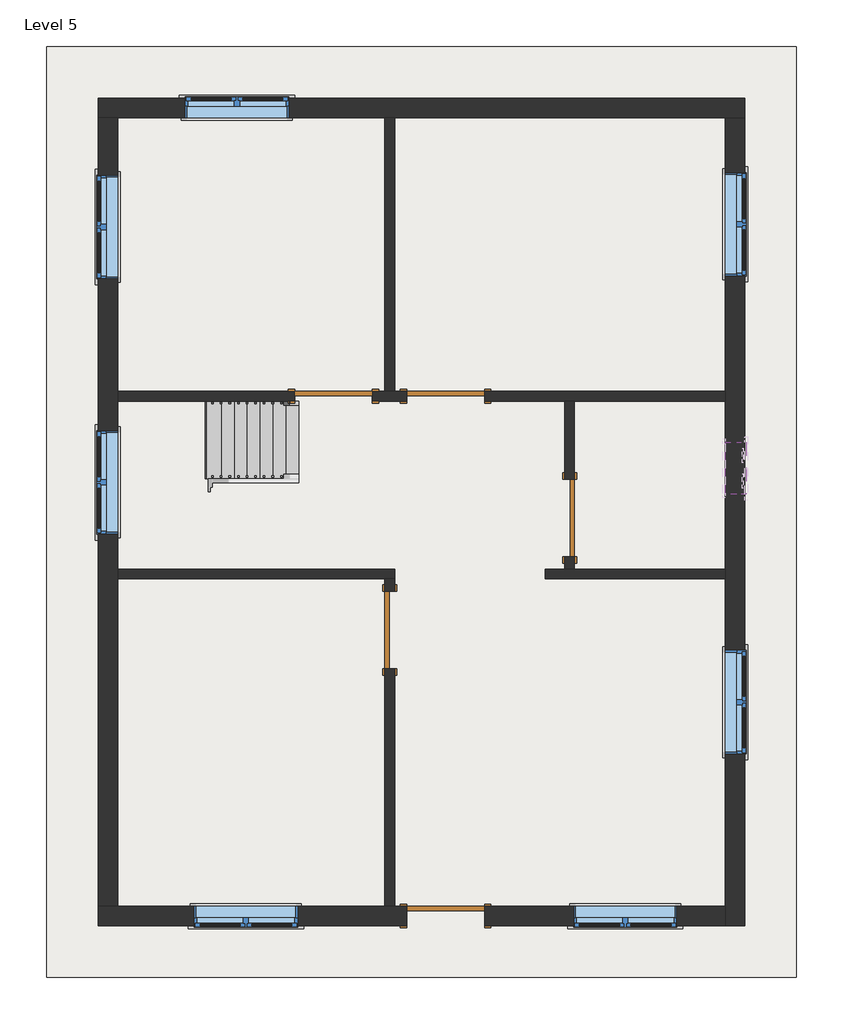
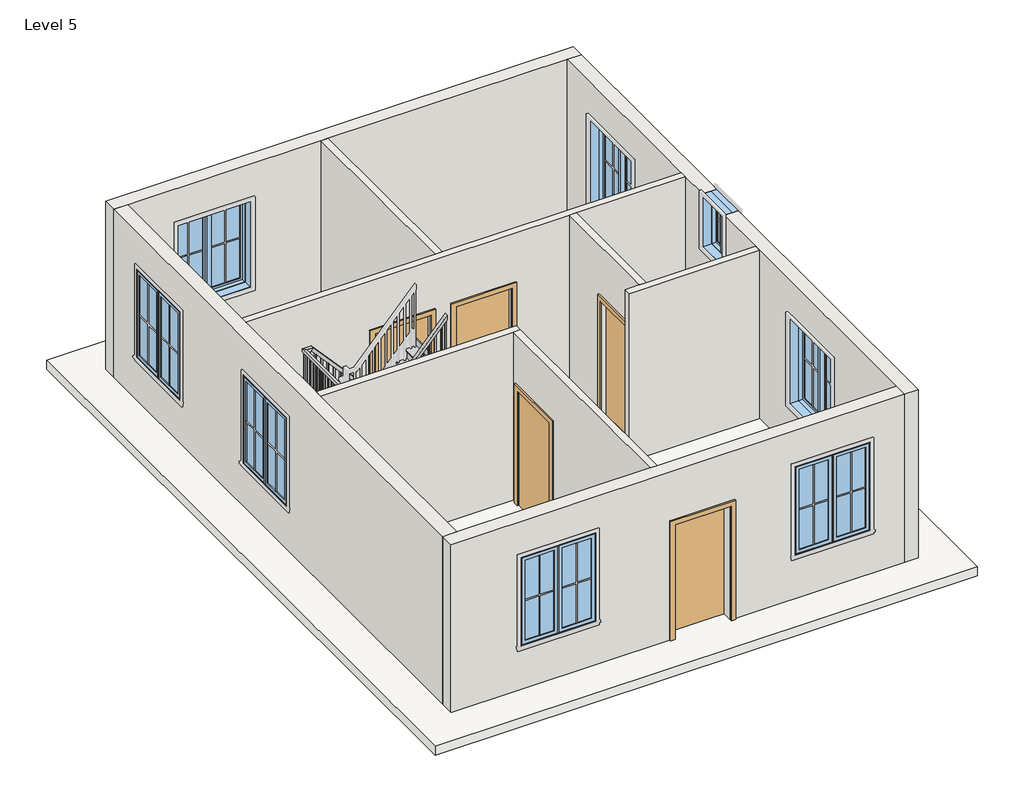
# One storey, part 1 of 2: 10 walls, 8 windows, 5 doors, 1 railing, 1 roof, 1 stair flight.
"""IFC4 building model written with IfcOpenShell, lengths in millimetres."""

from ifc_helpers import new_model, si_unit, frame, origin, place, context, project, spatial, polyline, outline, extrude, faceted_brep, transform, mapped, element, save
from components import door_e5f9f3c4, door_305aa2a5, door_a90ba1ad, stair_flight_93877f9a, window_c417fced, window_8377141f

model = new_model("IFC4")

# Units and contexts
model_context = context("Model", 3, world=origin())
ifc_project = project(units=[si_unit("LENGTHUNIT", "METRE", prefix="MILLI")], contexts=[model_context])

# Site, building, storey
site = spatial("IfcSite", under=ifc_project)
building = spatial("IfcBuilding", under=site)
storey = spatial("IfcBuildingStorey", under=building, Name="Level 5", Elevation=12192.0)

# Doors
placement = place(None, origin())
door_shape = door_e5f9f3c4(model_context)
element("IfcDoor", 1, ObjectType="Single-Flush : 36\" x 84\"", at=placement, inside=storey, context=model_context, shape_type="MappedRepresentation", body=[
    mapped(door_shape, transform((4044.95, 10966.45, 12192.0), x_axis=(1.0, 0.0, 0.0), y_axis=(0.0, 1.0, 0.0), z_axis=(0.0, 0.0, 1.0))),
])
element("IfcDoor", 2, ObjectType="Single-Flush : 36\" x 84\"", at=placement, inside=storey, context=model_context, shape_type="MappedRepresentation", body=[
    mapped(door_shape, transform((4705.35, 8210.55, 12192.0), x_axis=(0.0, 1.0, 0.0), y_axis=(-1.0, 0.0, 0.0), z_axis=(0.0, 0.0, 1.0))),
])
element("IfcDoor", 3, ObjectType="Single-Flush : 36\" x 84\"", at=placement, inside=storey, context=model_context, shape_type="MappedRepresentation", body=[
    mapped(door_shape, transform((6826.25, 9531.35, 12192.0), x_axis=(0.0, -1.0, 0.0), y_axis=(1.0, 0.0, 0.0), z_axis=(0.0, 0.0, 1.0))),
])
door_2_shape = door_305aa2a5(model_context)
element("IfcDoor", 4, ObjectType="Single-Flush : 36\" x 84\"", at=placement, inside=storey, context=model_context, shape_type="MappedRepresentation", body=[
    mapped(door_2_shape, transform((5365.75, 10966.45, 12192.0), x_axis=(-1.0, 0.0, 0.0), y_axis=(0.0, -1.0, 0.0), z_axis=(0.0, 0.0, 1.0))),
])
door_3_shape = door_a90ba1ad(model_context)
element("IfcDoor", 5, ObjectType="Single-Flush : 36\" x 84\"", at=placement, inside=storey, context=model_context, shape_type="MappedRepresentation", body=[
    mapped(door_3_shape, transform((5365.75, 4838.7, 12192.0), x_axis=(-1.0, 0.0, 0.0), y_axis=(0.0, -1.0, 0.0), z_axis=(0.0, 0.0, 1.0))),
])

# Railing
element("IfcRailing", 6, ObjectType="Handrail - Rectangular", at=placement, inside=storey, context=model_context, shape_type="SolidModel", body=[
    faceted_brep([(3632.2, 10858.5, 13275.7333333), (3632.2, 10858.5, 13199.7950998), (3632.2, 10909.3, 13199.7950998), (3632.2, 10909.3, 13275.7333333), (2565.4, 10858.5, 14461.0666667), (2542.7755898, 10858.5, 14410.2666667), (2542.7755898, 10909.3, 14410.2666667), (2565.4, 10909.3, 14461.0666667), (2463.8, 10858.5, 14461.0666667), (2463.8, 10858.5, 14410.2666667), (2413.0, 10909.3, 14410.2666667), (2413.0, 10909.3, 14461.0666667), (2463.8, 9055.1, 14461.0666667), (2463.8, 9004.3, 14410.2666667), (2413.0, 9004.3, 14410.2666667), (2413.0, 9055.1, 14461.0666667), (2463.8, 9055.1, 14602.1777778), (2463.8, 9004.3, 14551.3777778), (2413.0, 9004.3, 14551.3777778), (2413.0, 9055.1, 14602.1777778), (2463.8, 8978.9, 14602.1777778), (2463.8, 8978.9, 14551.3777778), (2413.0, 8928.1, 14551.3777778), (2413.0, 8928.1, 14602.1777778), (2540.0, 8978.9, 14602.1777778), (2562.6244102, 8978.9, 14551.3777778), (2562.6244102, 8928.1, 14551.3777778), (2540.0, 8928.1, 14602.1777778), (3632.2, 8978.9, 15815.7333333), (3632.2, 8928.1, 15815.7333333), (3632.2, 8928.1, 15739.7950998), (3632.2, 8978.9, 15739.7950998)], [[[0, 1, 2, 3]], [[1, 0, 4, 5]], [[2, 1, 5, 6]], [[3, 2, 6, 7]], [[0, 3, 7, 4]], [[5, 4, 8, 9]], [[6, 5, 9, 10]], [[7, 6, 10, 11]], [[4, 7, 11, 8]], [[9, 8, 12, 13]], [[10, 9, 13, 14]], [[11, 10, 14, 15]], [[8, 11, 15, 12]], [[13, 12, 16, 17]], [[14, 13, 17, 18]], [[15, 14, 18, 19]], [[12, 15, 19, 16]], [[17, 16, 20, 21]], [[18, 17, 21, 22]], [[19, 18, 22, 23]], [[16, 19, 23, 20]], [[21, 20, 24, 25]], [[22, 21, 25, 26]], [[23, 22, 26, 27]], [[20, 23, 27, 24]], [[28, 29, 30, 31]], [[25, 24, 28, 31]], [[26, 25, 31, 30]], [[27, 26, 30, 29]], [[24, 27, 29, 28]]]),
    extrude(outline(polyline([(15665.7117665, 3565.525), (15644.5450998, 3546.475), (14732.0, 3546.475), (14732.0, 3565.525), (15665.7117665, 3565.525)])), frame((0.0, 8943.975, 0.0), z_axis=(0.0, 1.0, 0.0), x_axis=(0.0, 0.0, 1.0)), (0.0, 0.0, 1.0), 19.05),
    extrude(outline(polyline([(15552.8228776, 3463.925), (15531.6562109, 3444.875), (14562.6666667, 3444.875), (14562.6666667, 3463.925), (15552.8228776, 3463.925)])), frame((0.0, 8943.975, 0.0), z_axis=(0.0, 1.0, 0.0), x_axis=(0.0, 0.0, 1.0)), (0.0, 0.0, 1.0), 19.05),
    extrude(outline(polyline([(15439.9339887, 3362.325), (15418.767322, 3343.275), (14562.6666667, 3343.275), (14562.6666667, 3362.325), (15439.9339887, 3362.325)])), frame((0.0, 8943.975, 0.0), z_axis=(0.0, 1.0, 0.0), x_axis=(0.0, 0.0, 1.0)), (0.0, 0.0, 1.0), 19.05),
    extrude(outline(polyline([(15327.0450998, 3260.725), (15305.8784332, 3241.675), (14393.3333333, 3241.675), (14393.3333333, 3260.725), (15327.0450998, 3260.725)])), frame((0.0, 8943.975, 0.0), z_axis=(0.0, 1.0, 0.0), x_axis=(0.0, 0.0, 1.0)), (0.0, 0.0, 1.0), 19.05),
    extrude(outline(polyline([(15214.1562109, 3159.125), (15192.9895443, 3140.075), (14224.0, 3140.075), (14224.0, 3159.125), (15214.1562109, 3159.125)])), frame((0.0, 8943.975, 0.0), z_axis=(0.0, 1.0, 0.0), x_axis=(0.0, 0.0, 1.0)), (0.0, 0.0, 1.0), 19.05),
    extrude(outline(polyline([(15101.267322, 3057.525), (15080.1006554, 3038.475), (14224.0, 3038.475), (14224.0, 3057.525), (15101.267322, 3057.525)])), frame((0.0, 8943.975, 0.0), z_axis=(0.0, 1.0, 0.0), x_axis=(0.0, 0.0, 1.0)), (0.0, 0.0, 1.0), 19.05),
    extrude(outline(polyline([(14988.3784332, 2955.925), (14967.2117665, 2936.875), (14054.6666667, 2936.875), (14054.6666667, 2955.925), (14988.3784332, 2955.925)])), frame((0.0, 8943.975, 0.0), z_axis=(0.0, 1.0, 0.0), x_axis=(0.0, 0.0, 1.0)), (0.0, 0.0, 1.0), 19.05),
    extrude(outline(polyline([(14875.4895443, 2854.325), (14854.3228776, 2835.275), (13885.3333333, 2835.275), (13885.3333333, 2854.325), (14875.4895443, 2854.325)])), frame((0.0, 8943.975, 0.0), z_axis=(0.0, 1.0, 0.0), x_axis=(0.0, 0.0, 1.0)), (0.0, 0.0, 1.0), 19.05),
    extrude(outline(polyline([(14762.6006554, 2752.725), (14741.4339887, 2733.675), (13885.3333333, 2733.675), (13885.3333333, 2752.725), (14762.6006554, 2752.725)])), frame((0.0, 8943.975, 0.0), z_axis=(0.0, 1.0, 0.0), x_axis=(0.0, 0.0, 1.0)), (0.0, 0.0, 1.0), 19.05),
    extrude(outline(polyline([(14649.7117665, 2651.125), (14628.5450998, 2632.075), (13716.0, 2632.075), (13716.0, 2651.125), (14649.7117665, 2651.125)])), frame((0.0, 8943.975, 0.0), z_axis=(0.0, 1.0, 0.0), x_axis=(0.0, 0.0, 1.0)), (0.0, 0.0, 1.0), 19.05),
    extrude(outline(polyline([(14536.8228776, 2549.525), (14515.6562109, 2530.475), (13546.6666667, 2530.475), (13546.6666667, 2549.525), (14536.8228776, 2549.525)])), frame((0.0, 8943.975, 0.0), z_axis=(0.0, 1.0, 0.0), x_axis=(0.0, 0.0, 1.0)), (0.0, 0.0, 1.0), 19.05),
    extrude(outline(polyline([(2428.875, 9064.625), (2447.925, 9064.625), (2447.925, 9045.575), (2428.875, 9045.575), (2428.875, 9064.625)])), frame((0.0, 0.0, 13546.6666667), z_axis=(0.0, 0.0, 1.0), x_axis=(1.0, 0.0, 0.0)), (0.0, 0.0, 1.0), 863.6),
    extrude(outline(polyline([(2428.875, 9166.225), (2447.925, 9166.225), (2447.925, 9147.175), (2428.875, 9147.175), (2428.875, 9166.225)])), frame((0.0, 0.0, 13546.6666667), z_axis=(0.0, 0.0, 1.0), x_axis=(1.0, 0.0, 0.0)), (0.0, 0.0, 1.0), 863.6),
    extrude(outline(polyline([(2428.875, 9267.825), (2447.925, 9267.825), (2447.925, 9248.775), (2428.875, 9248.775), (2428.875, 9267.825)])), frame((0.0, 0.0, 13546.6666667), z_axis=(0.0, 0.0, 1.0), x_axis=(1.0, 0.0, 0.0)), (0.0, 0.0, 1.0), 863.6),
    extrude(outline(polyline([(2428.875, 9369.425), (2447.925, 9369.425), (2447.925, 9350.375), (2428.875, 9350.375), (2428.875, 9369.425)])), frame((0.0, 0.0, 13546.6666667), z_axis=(0.0, 0.0, 1.0), x_axis=(1.0, 0.0, 0.0)), (0.0, 0.0, 1.0), 863.6),
    extrude(outline(polyline([(2428.875, 9471.025), (2447.925, 9471.025), (2447.925, 9451.975), (2428.875, 9451.975), (2428.875, 9471.025)])), frame((0.0, 0.0, 13546.6666667), z_axis=(0.0, 0.0, 1.0), x_axis=(1.0, 0.0, 0.0)), (0.0, 0.0, 1.0), 863.6),
    extrude(outline(polyline([(2428.875, 9572.625), (2447.925, 9572.625), (2447.925, 9553.575), (2428.875, 9553.575), (2428.875, 9572.625)])), frame((0.0, 0.0, 13546.6666667), z_axis=(0.0, 0.0, 1.0), x_axis=(1.0, 0.0, 0.0)), (0.0, 0.0, 1.0), 863.6),
    extrude(outline(polyline([(2428.875, 9674.225), (2447.925, 9674.225), (2447.925, 9655.175), (2428.875, 9655.175), (2428.875, 9674.225)])), frame((0.0, 0.0, 13546.6666667), z_axis=(0.0, 0.0, 1.0), x_axis=(1.0, 0.0, 0.0)), (0.0, 0.0, 1.0), 863.6),
    extrude(outline(polyline([(2428.875, 9775.825), (2447.925, 9775.825), (2447.925, 9756.775), (2428.875, 9756.775), (2428.875, 9775.825)])), frame((0.0, 0.0, 13546.6666667), z_axis=(0.0, 0.0, 1.0), x_axis=(1.0, 0.0, 0.0)), (0.0, 0.0, 1.0), 863.6),
    extrude(outline(polyline([(2428.875, 9877.425), (2447.925, 9877.425), (2447.925, 9858.375), (2428.875, 9858.375), (2428.875, 9877.425)])), frame((0.0, 0.0, 13546.6666667), z_axis=(0.0, 0.0, 1.0), x_axis=(1.0, 0.0, 0.0)), (0.0, 0.0, 1.0), 863.6),
    extrude(outline(polyline([(2428.875, 9979.025), (2447.925, 9979.025), (2447.925, 9959.975), (2428.875, 9959.975), (2428.875, 9979.025)])), frame((0.0, 0.0, 13546.6666667), z_axis=(0.0, 0.0, 1.0), x_axis=(1.0, 0.0, 0.0)), (0.0, 0.0, 1.0), 863.6),
    extrude(outline(polyline([(2428.875, 10080.625), (2447.925, 10080.625), (2447.925, 10061.575), (2428.875, 10061.575), (2428.875, 10080.625)])), frame((0.0, 0.0, 13546.6666667), z_axis=(0.0, 0.0, 1.0), x_axis=(1.0, 0.0, 0.0)), (0.0, 0.0, 1.0), 863.6),
    extrude(outline(polyline([(2428.875, 10182.225), (2447.925, 10182.225), (2447.925, 10163.175), (2428.875, 10163.175), (2428.875, 10182.225)])), frame((0.0, 0.0, 13546.6666667), z_axis=(0.0, 0.0, 1.0), x_axis=(1.0, 0.0, 0.0)), (0.0, 0.0, 1.0), 863.6),
    extrude(outline(polyline([(2428.875, 10283.825), (2447.925, 10283.825), (2447.925, 10264.775), (2428.875, 10264.775), (2428.875, 10283.825)])), frame((0.0, 0.0, 13546.6666667), z_axis=(0.0, 0.0, 1.0), x_axis=(1.0, 0.0, 0.0)), (0.0, 0.0, 1.0), 863.6),
    extrude(outline(polyline([(2428.875, 10385.425), (2447.925, 10385.425), (2447.925, 10366.375), (2428.875, 10366.375), (2428.875, 10385.425)])), frame((0.0, 0.0, 13546.6666667), z_axis=(0.0, 0.0, 1.0), x_axis=(1.0, 0.0, 0.0)), (0.0, 0.0, 1.0), 863.6),
    extrude(outline(polyline([(2428.875, 10487.025), (2447.925, 10487.025), (2447.925, 10467.975), (2428.875, 10467.975), (2428.875, 10487.025)])), frame((0.0, 0.0, 13546.6666667), z_axis=(0.0, 0.0, 1.0), x_axis=(1.0, 0.0, 0.0)), (0.0, 0.0, 1.0), 863.6),
    extrude(outline(polyline([(2428.875, 10588.625), (2447.925, 10588.625), (2447.925, 10569.575), (2428.875, 10569.575), (2428.875, 10588.625)])), frame((0.0, 0.0, 13546.6666667), z_axis=(0.0, 0.0, 1.0), x_axis=(1.0, 0.0, 0.0)), (0.0, 0.0, 1.0), 863.6),
    extrude(outline(polyline([(2428.875, 10690.225), (2447.925, 10690.225), (2447.925, 10671.175), (2428.875, 10671.175), (2428.875, 10690.225)])), frame((0.0, 0.0, 13546.6666667), z_axis=(0.0, 0.0, 1.0), x_axis=(1.0, 0.0, 0.0)), (0.0, 0.0, 1.0), 863.6),
    extrude(outline(polyline([(2428.875, 10791.825), (2447.925, 10791.825), (2447.925, 10772.775), (2428.875, 10772.775), (2428.875, 10791.825)])), frame((0.0, 0.0, 13546.6666667), z_axis=(0.0, 0.0, 1.0), x_axis=(1.0, 0.0, 0.0)), (0.0, 0.0, 1.0), 863.6),
    extrude(outline(polyline([(2524.125, 10893.425), (2524.125, 10874.375), (2505.075, 10874.375), (2505.075, 10893.425), (2524.125, 10893.425)])), frame((0.0, 0.0, 13546.6666667), z_axis=(0.0, 0.0, 1.0), x_axis=(1.0, 0.0, 0.0)), (0.0, 0.0, 1.0), 863.6),
    extrude(outline(polyline([(14318.1006554, 2625.725), (14339.267322, 2606.675), (13377.3333333, 2606.675), (13377.3333333, 2625.725), (14318.1006554, 2625.725)])), frame((0.0, 10874.375, 0.0), z_axis=(0.0, 1.0, 0.0), x_axis=(0.0, 0.0, 1.0)), (0.0, 0.0, 1.0), 19.05),
    extrude(outline(polyline([(14205.2117665, 2727.325), (14226.3784332, 2708.275), (13377.3333333, 2708.275), (13377.3333333, 2727.325), (14205.2117665, 2727.325)])), frame((0.0, 10874.375, 0.0), z_axis=(0.0, 1.0, 0.0), x_axis=(0.0, 0.0, 1.0)), (0.0, 0.0, 1.0), 19.05),
    extrude(outline(polyline([(14092.3228776, 2828.925), (14113.4895443, 2809.875), (13208.0, 2809.875), (13208.0, 2828.925), (14092.3228776, 2828.925)])), frame((0.0, 10874.375, 0.0), z_axis=(0.0, 1.0, 0.0), x_axis=(0.0, 0.0, 1.0)), (0.0, 0.0, 1.0), 19.05),
    extrude(outline(polyline([(13979.4339887, 2930.525), (14000.6006554, 2911.475), (13038.6666667, 2911.475), (13038.6666667, 2930.525), (13979.4339887, 2930.525)])), frame((0.0, 10874.375, 0.0), z_axis=(0.0, 1.0, 0.0), x_axis=(0.0, 0.0, 1.0)), (0.0, 0.0, 1.0), 19.05),
    extrude(outline(polyline([(13866.5450998, 3032.125), (13887.7117665, 3013.075), (13038.6666667, 3013.075), (13038.6666667, 3032.125), (13866.5450998, 3032.125)])), frame((0.0, 10874.375, 0.0), z_axis=(0.0, 1.0, 0.0), x_axis=(0.0, 0.0, 1.0)), (0.0, 0.0, 1.0), 19.05),
    extrude(outline(polyline([(13753.6562109, 3133.725), (13774.8228776, 3114.675), (12869.3333333, 3114.675), (12869.3333333, 3133.725), (13753.6562109, 3133.725)])), frame((0.0, 10874.375, 0.0), z_axis=(0.0, 1.0, 0.0), x_axis=(0.0, 0.0, 1.0)), (0.0, 0.0, 1.0), 19.05),
    extrude(outline(polyline([(13640.767322, 3235.325), (13661.9339887, 3216.275), (12700.0, 3216.275), (12700.0, 3235.325), (13640.767322, 3235.325)])), frame((0.0, 10874.375, 0.0), z_axis=(0.0, 1.0, 0.0), x_axis=(0.0, 0.0, 1.0)), (0.0, 0.0, 1.0), 19.05),
    extrude(outline(polyline([(13527.8784332, 3336.925), (13549.0450998, 3317.875), (12700.0, 3317.875), (12700.0, 3336.925), (13527.8784332, 3336.925)])), frame((0.0, 10874.375, 0.0), z_axis=(0.0, 1.0, 0.0), x_axis=(0.0, 0.0, 1.0)), (0.0, 0.0, 1.0), 19.05),
    extrude(outline(polyline([(13414.9895443, 3438.525), (13436.1562109, 3419.475), (12530.6666667, 3419.475), (12530.6666667, 3438.525), (13414.9895443, 3438.525)])), frame((0.0, 10874.375, 0.0), z_axis=(0.0, 1.0, 0.0), x_axis=(0.0, 0.0, 1.0)), (0.0, 0.0, 1.0), 19.05),
    extrude(outline(polyline([(13302.1006554, 3540.125), (13323.267322, 3521.075), (12361.3333333, 3521.075), (12361.3333333, 3540.125), (13302.1006554, 3540.125)])), frame((0.0, 10874.375, 0.0), z_axis=(0.0, 1.0, 0.0), x_axis=(0.0, 0.0, 1.0)), (0.0, 0.0, 1.0), 19.05),
    extrude(outline(polyline([(2428.875, 8963.025), (2447.925, 8963.025), (2447.925, 8943.975), (2428.875, 8943.975), (2428.875, 8963.025)])), frame((0.0, 0.0, 13546.6666667), z_axis=(0.0, 0.0, 1.0), x_axis=(1.0, 0.0, 0.0)), (0.0, 0.0, 1.0), 1004.7111111),
    extrude(outline(polyline([(2447.925, 10893.425), (2447.925, 10874.375), (2428.875, 10874.375), (2428.875, 10893.425), (2447.925, 10893.425)])), frame((0.0, 0.0, 13546.6666667), z_axis=(0.0, 0.0, 1.0), x_axis=(1.0, 0.0, 0.0)), (0.0, 0.0, 1.0), 863.6),
    extrude(outline(polyline([(15739.7950998, 3632.2), (15718.6284332, 3613.15), (14732.0, 3613.15), (14732.0, 3632.2), (15739.7950998, 3632.2)])), frame((0.0, 8943.975, 0.0), z_axis=(0.0, 1.0, 0.0), x_axis=(0.0, 0.0, 1.0)), (0.0, 0.0, 1.0), 19.05),
    extrude(outline(polyline([(13199.7950998, 3632.2), (13220.9617665, 3613.15), (12361.3333333, 3613.15), (12361.3333333, 3632.2), (13199.7950998, 3632.2)])), frame((0.0, 10874.375, 0.0), z_axis=(0.0, 1.0, 0.0), x_axis=(0.0, 0.0, 1.0)), (0.0, 0.0, 1.0), 19.05),
])

# Roof
element("IfcRoof", 7, ObjectType="Generic - 12\"", at=placement, inside=storey, context=model_context, shape_type="SweptSolid", body=[
    extrude(outline(polyline([(660.4, 15087.6), (9499.6, 15087.6), (9499.6, 4114.8), (660.4, 4114.8), (660.4, 15087.6)])), frame((0.0, 0.0, 12192.0), z_axis=(0.0, 0.0, 1.0), x_axis=(1.0, 0.0, 0.0)), (0.0, 0.0, 1.0), 152.4),
])

# Stair flight
stair_flight_shape = stair_flight_93877f9a(model_context)
element("IfcStairFlight", 8, ObjectType="2\" Tread 1\" Nosing 1/4\" Riser", at=placement, inside=storey, context=model_context, shape_type="MappedRepresentation", body=[
    mapped(stair_flight_shape, transform((0.0, 0.0, 0.0), x_axis=(1.0, 0.0, 0.0), y_axis=(0.0, 1.0, 0.0), z_axis=(0.0, 0.0, 1.0))),
])

# Walls
element("IfcWall", 9, ObjectType="Generic - 5\"", at=placement, inside=storey, context=model_context, shape_type="SweptSolid", body=[
    extrude(outline(polyline([(4648.2, 11023.6), (4648.2, 14249.4), (4762.5, 14249.4), (4762.5, 11023.6), (4648.2, 11023.6)])), frame((0.0, 0.0, 12192.0), z_axis=(0.0, 0.0, 1.0), x_axis=(1.0, 0.0, 0.0)), (0.0, 0.0, 1.0), 3048.0),
])
element("IfcWall", 10, ObjectType="Generic - 5\"", at=placement, inside=storey, context=model_context, shape_type="Brep", body=[
    faceted_brep([(4502.15, 10909.3, 12192.0), (4908.55, 10909.3, 12192.0), (4908.55, 10909.3, 14325.6), (5822.95, 10909.3, 14325.6), (5822.95, 10909.3, 12192.0), (6769.1, 10909.3, 12192.0), (6883.4, 10909.3, 12192.0), (8661.4, 10909.3, 12192.0), (8661.4, 10909.3, 15240.0), (6883.4, 10909.3, 15240.0), (6769.1, 10909.3, 15240.0), (1498.6, 10909.3, 15240.0), (1498.6, 10909.3, 12192.0), (3587.75, 10909.3, 12192.0), (3587.75, 10909.3, 14325.6), (4502.15, 10909.3, 14325.6), (4908.55, 11023.6, 14325.6), (4908.55, 11023.6, 12192.0), (4762.5, 11023.6, 12192.0), (4648.2, 11023.6, 12192.0), (4502.15, 11023.6, 12192.0), (4502.15, 11023.6, 14325.6), (3587.75, 11023.6, 14325.6), (3587.75, 11023.6, 12192.0), (1498.6, 11023.6, 12192.0), (1498.6, 11023.6, 15240.0), (4648.2, 11023.6, 15240.0), (4762.5, 11023.6, 15240.0), (8661.4, 11023.6, 15240.0), (8661.4, 11023.6, 12192.0), (5822.95, 11023.6, 12192.0), (5822.95, 11023.6, 14325.6)], [[[0, 1, 2, 3, 4, 5, 6, 7, 8, 9, 10, 11, 12, 13, 14, 15]], [[16, 17, 18, 19, 20, 21, 22, 23, 24, 25, 26, 27, 28, 29, 30, 31]], [[13, 12, 24, 23]], [[30, 29, 7, 6, 5, 4]], [[20, 19, 18, 17, 1, 0]], [[11, 10, 9, 8, 28, 27, 26, 25]], [[8, 7, 29, 28]], [[12, 11, 25, 24]], [[21, 20, 0, 15]], [[22, 21, 15, 14]], [[23, 22, 14, 13]], [[2, 1, 17, 16]], [[3, 2, 16, 31]], [[4, 3, 31, 30]]]),
])
element("IfcWall", 11, ObjectType="Generic - 5\"", at=placement, inside=storey, context=model_context, shape_type="SweptSolid", body=[
    extrude(outline(polyline([(9074.15, 14325.6), (9074.15, 12192.0), (8928.1, 12192.0), (8928.1, 15240.0), (10909.3, 15240.0), (10909.3, 12192.0), (9988.55, 12192.0), (9988.55, 14325.6), (9074.15, 14325.6)])), frame((6769.1, 0.0, 0.0), z_axis=(1.0, 0.0, 0.0), x_axis=(0.0, 1.0, 0.0)), (0.0, 0.0, 1.0), 114.3),
])
element("IfcWall", 12, ObjectType="Generic - 5\"", at=placement, inside=storey, context=model_context, shape_type="Brep", body=[
    faceted_brep([(1498.6, 8813.8, 12192.0), (4648.2, 8813.8, 12192.0), (4762.5, 8813.8, 12192.0), (4762.5, 8813.8, 15240.0), (4648.2, 8813.8, 15240.0), (1498.6, 8813.8, 15240.0), (1498.6, 8928.1, 12192.0), (1498.6, 8928.1, 15240.0), (4762.5, 8928.1, 15240.0), (4762.5, 8928.1, 12192.0)], [[[0, 1, 2, 3, 4, 5]], [[6, 7, 8, 9]], [[2, 1, 0, 6, 9]], [[5, 4, 3, 8, 7]], [[0, 5, 7, 6]], [[3, 2, 9, 8]]]),
])
element("IfcWall", 13, ObjectType="Generic - 5\"", at=placement, inside=storey, context=model_context, shape_type="SweptSolid", body=[
    extrude(outline(polyline([(8813.8, 12192.0), (8667.75, 12192.0), (8667.75, 14325.6), (7753.35, 14325.6), (7753.35, 12192.0), (4953.0, 12192.0), (4953.0, 15240.0), (8813.8, 15240.0), (8813.8, 12192.0)])), frame((4648.2, 0.0, 0.0), z_axis=(1.0, 0.0, 0.0), x_axis=(0.0, 1.0, 0.0)), (0.0, 0.0, 1.0), 114.3),
])
element("IfcWall", 14, ObjectType="Generic - 5\"", at=placement, inside=storey, context=model_context, shape_type="Brep", body=[
    faceted_brep([(6540.5050896, 8813.8, 12192.0), (8661.4, 8813.8, 12192.0), (8661.4, 8813.8, 15240.0), (6540.5050896, 8813.8, 15240.0), (6540.5050896, 8928.1, 12192.0), (6540.5050896, 8928.1, 15240.0), (6769.1, 8928.1, 15240.0), (6883.4, 8928.1, 15240.0), (8661.4, 8928.1, 15240.0), (8661.4, 8928.1, 12192.0), (6883.4, 8928.1, 12192.0), (6769.1, 8928.1, 12192.0)], [[[0, 1, 2, 3]], [[4, 5, 6, 7, 8, 9, 10, 11]], [[1, 0, 4, 11, 10, 9]], [[3, 2, 8, 7, 6, 5]], [[0, 3, 5, 4]], [[2, 1, 9, 8]]]),
])
element("IfcWall", 15, ObjectType="Generic - 8\"", at=placement, inside=storey, context=model_context, shape_type="Brep", body=[
    faceted_brep([(1270.0, 14249.4, 12192.0), (1498.6, 14249.4, 12192.0), (4648.2, 14249.4, 12192.0), (4762.5, 14249.4, 12192.0), (8661.4, 14249.4, 12192.0), (8890.0, 14249.4, 12192.0), (8890.0, 14249.4, 15240.0), (8661.4, 14249.4, 15240.0), (4762.5, 14249.4, 15240.0), (4648.2, 14249.4, 15240.0), (1498.6, 14249.4, 15240.0), (1270.0, 14249.4, 15240.0), (3514.725, 14249.4, 14630.4), (3514.725, 14249.4, 13106.4), (2295.525, 14249.4, 13106.4), (2295.525, 14249.4, 14630.4), (1270.0, 14478.0, 12192.0), (1270.0, 14478.0, 15240.0), (8890.0, 14478.0, 15240.0), (8890.0, 14478.0, 12192.0), (3514.725, 14478.0, 14630.4), (2295.525, 14478.0, 14630.4), (2295.525, 14478.0, 13106.4), (3514.725, 14478.0, 13106.4)], [[[0, 1, 2, 3, 4, 5, 6, 7, 8, 9, 10, 11], [12, 13, 14, 15]], [[16, 17, 18, 19], [20, 21, 22, 23]], [[5, 4, 3, 2, 1, 0, 16, 19]], [[11, 10, 9, 8, 7, 6, 18, 17]], [[6, 5, 19, 18]], [[0, 11, 17, 16]], [[13, 12, 20, 23]], [[14, 13, 23, 22]], [[15, 14, 22, 21]], [[12, 15, 21, 20]]]),
])
element("IfcWall", 16, ObjectType="Generic - 8\"", at=placement, inside=storey, context=model_context, shape_type="Brep", body=[
    faceted_brep([(8661.4, 14249.4, 12192.0), (8661.4, 11023.6, 12192.0), (8661.4, 10909.3, 12192.0), (8661.4, 8928.1, 12192.0), (8661.4, 8813.8, 12192.0), (8661.4, 4953.0, 12192.0), (8661.4, 4724.4, 12192.0), (8661.4, 4724.4, 15240.0), (8661.4, 4953.0, 15240.0), (8661.4, 8813.8, 15240.0), (8661.4, 8928.1, 15240.0), (8661.4, 9810.75, 15240.0), (8661.4, 9810.75, 14325.6), (8661.4, 10420.35, 14325.6), (8661.4, 10420.35, 15240.0), (8661.4, 10909.3, 15240.0), (8661.4, 11023.6, 15240.0), (8661.4, 14249.4, 15240.0), (8661.4, 6750.05, 14630.4), (8661.4, 6750.05, 13106.4), (8661.4, 7969.25, 13106.4), (8661.4, 7969.25, 14630.4), (8661.4, 12382.5, 14630.4), (8661.4, 12382.5, 13106.4), (8661.4, 13601.7, 13106.4), (8661.4, 13601.7, 14630.4), (8890.0, 4724.4, 12192.0), (8890.0, 14249.4, 12192.0), (8890.0, 14249.4, 15240.0), (8890.0, 10420.35, 15240.0), (8890.0, 10420.35, 14325.6), (8890.0, 9810.75, 14325.6), (8890.0, 9810.75, 15240.0), (8890.0, 4724.4, 15240.0), (8890.0, 6750.05, 13106.4), (8890.0, 6750.05, 14630.4), (8890.0, 7969.25, 14630.4), (8890.0, 7969.25, 13106.4), (8890.0, 12382.5, 13106.4), (8890.0, 12382.5, 14630.4), (8890.0, 13601.7, 14630.4), (8890.0, 13601.7, 13106.4)], [[[0, 1, 2, 3, 4, 5, 6, 7, 8, 9, 10, 11, 12, 13, 14, 15, 16, 17], [18, 19, 20, 21], [22, 23, 24, 25]], [[26, 27, 28, 29, 30, 31, 32, 33], [34, 35, 36, 37], [38, 39, 40, 41]], [[6, 5, 4, 3, 2, 1, 0, 27, 26]], [[28, 17, 16, 15, 14, 29]], [[7, 33, 32, 11, 10, 9, 8]], [[0, 17, 28, 27]], [[7, 6, 26, 33]], [[19, 18, 35, 34]], [[20, 19, 34, 37]], [[21, 20, 37, 36]], [[18, 21, 36, 35]], [[23, 22, 39, 38]], [[24, 23, 38, 41]], [[25, 24, 41, 40]], [[22, 25, 40, 39]], [[31, 12, 11, 32]], [[12, 31, 30, 13]], [[13, 30, 29, 14]]]),
])
element("IfcWall", 17, ObjectType="Generic - 8\"", at=placement, inside=storey, context=model_context, shape_type="Brep", body=[
    faceted_brep([(4908.55, 4953.0, 14325.6), (4908.55, 4953.0, 12192.0), (4762.5, 4953.0, 12192.0), (4648.2, 4953.0, 12192.0), (1498.6, 4953.0, 12192.0), (1270.0, 4953.0, 12192.0), (1270.0, 4953.0, 15240.0), (1498.6, 4953.0, 15240.0), (4648.2, 4953.0, 15240.0), (4762.5, 4953.0, 15240.0), (8661.4, 4953.0, 15240.0), (8661.4, 4953.0, 12192.0), (5822.95, 4953.0, 12192.0), (5822.95, 4953.0, 14325.6), (2400.3, 4953.0, 14630.4), (2400.3, 4953.0, 13106.4), (3619.5, 4953.0, 13106.4), (3619.5, 4953.0, 14630.4), (6872.2875, 4953.0, 14630.4), (6872.2875, 4953.0, 13106.4), (8091.4875, 4953.0, 13106.4), (8091.4875, 4953.0, 14630.4), (1270.0, 4724.4, 12192.0), (4908.55, 4724.4, 12192.0), (4908.55, 4724.4, 14325.6), (5822.95, 4724.4, 14325.6), (5822.95, 4724.4, 12192.0), (8661.4, 4724.4, 12192.0), (8661.4, 4724.4, 15240.0), (1270.0, 4724.4, 15240.0), (2400.3, 4724.4, 14630.4), (3619.5, 4724.4, 14630.4), (3619.5, 4724.4, 13106.4), (2400.3, 4724.4, 13106.4), (6872.2875, 4724.4, 14630.4), (8091.4875, 4724.4, 14630.4), (8091.4875, 4724.4, 13106.4), (6872.2875, 4724.4, 13106.4)], [[[0, 1, 2, 3, 4, 5, 6, 7, 8, 9, 10, 11, 12, 13], [14, 15, 16, 17], [18, 19, 20, 21]], [[22, 23, 24, 25, 26, 27, 28, 29], [30, 31, 32, 33], [34, 35, 36, 37]], [[12, 11, 27, 26]], [[5, 4, 3, 2, 1, 23, 22]], [[10, 9, 8, 7, 6, 29, 28]], [[11, 10, 28, 27]], [[6, 5, 22, 29]], [[24, 23, 1, 0]], [[25, 24, 0, 13]], [[26, 25, 13, 12]], [[15, 14, 30, 33]], [[16, 15, 33, 32]], [[17, 16, 32, 31]], [[14, 17, 31, 30]], [[19, 18, 34, 37]], [[20, 19, 37, 36]], [[21, 20, 36, 35]], [[18, 21, 35, 34]]]),
])
element("IfcWall", 18, ObjectType="Generic - 8\"", at=placement, inside=storey, context=model_context, shape_type="Brep", body=[
    faceted_brep([(1498.6, 4953.0, 12192.0), (1498.6, 8813.8, 12192.0), (1498.6, 8928.1, 12192.0), (1498.6, 10909.3, 12192.0), (1498.6, 11023.6, 12192.0), (1498.6, 14249.4, 12192.0), (1498.6, 14249.4, 15240.0), (1498.6, 11023.6, 15240.0), (1498.6, 10909.3, 15240.0), (1498.6, 8928.1, 15240.0), (1498.6, 8813.8, 15240.0), (1498.6, 4953.0, 15240.0), (1498.6, 13569.95, 14630.4), (1498.6, 13569.95, 13106.4), (1498.6, 12350.75, 13106.4), (1498.6, 12350.75, 14630.4), (1498.6, 10560.05, 14630.4), (1498.6, 10560.05, 13106.4), (1498.6, 9340.85, 13106.4), (1498.6, 9340.85, 14630.4), (1270.0, 14249.4, 12192.0), (1270.0, 4953.0, 12192.0), (1270.0, 4953.0, 15240.0), (1270.0, 14249.4, 15240.0), (1270.0, 13569.95, 13106.4), (1270.0, 13569.95, 14630.4), (1270.0, 12350.75, 14630.4), (1270.0, 12350.75, 13106.4), (1270.0, 10560.05, 13106.4), (1270.0, 10560.05, 14630.4), (1270.0, 9340.85, 14630.4), (1270.0, 9340.85, 13106.4)], [[[0, 1, 2, 3, 4, 5, 6, 7, 8, 9, 10, 11], [12, 13, 14, 15], [16, 17, 18, 19]], [[20, 21, 22, 23], [24, 25, 26, 27], [28, 29, 30, 31]], [[5, 4, 3, 2, 1, 0, 21, 20]], [[11, 10, 9, 8, 7, 6, 23, 22]], [[6, 5, 20, 23]], [[0, 11, 22, 21]], [[13, 12, 25, 24]], [[14, 13, 24, 27]], [[15, 14, 27, 26]], [[12, 15, 26, 25]], [[17, 16, 29, 28]], [[18, 17, 28, 31]], [[19, 18, 31, 30]], [[16, 19, 30, 29]]]),
])

# Windows
window_shape = window_c417fced(model_context)
element("IfcWindow", 19, ObjectType="Window-Casement-Double : 24\" x 36\"", at=placement, inside=storey, context=model_context, shape_type="MappedRepresentation", body=[
    mapped(window_shape, transform((8775.7, 10115.55, 13411.2), x_axis=(0.0, -1.0, 0.0), y_axis=(1.0, 0.0, 0.0), z_axis=(0.0, 0.0, 1.0))),
])
window_2_shape = window_8377141f(model_context)
element("IfcWindow", 20, ObjectType="Window-Casement-Double : 48\" x 60\"", at=placement, inside=storey, context=model_context, shape_type="MappedRepresentation", body=[
    mapped(window_2_shape, transform((7481.8875, 4838.7, 12192.0), x_axis=(-1.0, 0.0, 0.0), y_axis=(0.0, -1.0, 0.0), z_axis=(0.0, 0.0, 1.0))),
])
element("IfcWindow", 21, ObjectType="Window-Casement-Double : 48\" x 60\"", at=placement, inside=storey, context=model_context, shape_type="MappedRepresentation", body=[
    mapped(window_2_shape, transform((3009.9, 4838.7, 12192.0), x_axis=(-1.0, 0.0, 0.0), y_axis=(0.0, -1.0, 0.0), z_axis=(0.0, 0.0, 1.0))),
])
element("IfcWindow", 22, ObjectType="Window-Casement-Double : 48\" x 60\"", at=placement, inside=storey, context=model_context, shape_type="MappedRepresentation", body=[
    mapped(window_2_shape, transform((8775.7, 12992.1, 12192.0), x_axis=(0.0, -1.0, 0.0), y_axis=(1.0, 0.0, 0.0), z_axis=(0.0, 0.0, 1.0))),
])
element("IfcWindow", 23, ObjectType="Window-Casement-Double : 48\" x 60\"", at=placement, inside=storey, context=model_context, shape_type="MappedRepresentation", body=[
    mapped(window_2_shape, transform((8775.7, 7359.65, 12192.0), x_axis=(0.0, -1.0, 0.0), y_axis=(1.0, 0.0, 0.0), z_axis=(0.0, 0.0, 1.0))),
])
element("IfcWindow", 24, ObjectType="Window-Casement-Double : 48\" x 60\"", at=placement, inside=storey, context=model_context, shape_type="MappedRepresentation", body=[
    mapped(window_2_shape, transform((1384.3, 12960.35, 12192.0), x_axis=(0.0, 1.0, 0.0), y_axis=(-1.0, 0.0, 0.0), z_axis=(0.0, 0.0, 1.0))),
])
element("IfcWindow", 25, ObjectType="Window-Casement-Double : 48\" x 60\"", at=placement, inside=storey, context=model_context, shape_type="MappedRepresentation", body=[
    mapped(window_2_shape, transform((1384.3, 9950.45, 12192.0), x_axis=(0.0, 1.0, 0.0), y_axis=(-1.0, 0.0, 0.0), z_axis=(0.0, 0.0, 1.0))),
])
element("IfcWindow", 26, ObjectType="Window-Casement-Double : 48\" x 60\"", at=placement, inside=storey, context=model_context, shape_type="MappedRepresentation", body=[
    mapped(window_2_shape, transform((2905.125, 14363.7, 12192.0), x_axis=(1.0, 0.0, 0.0), y_axis=(0.0, 1.0, 0.0), z_axis=(0.0, 0.0, 1.0))),
])

save(model, "model.ifc")

# Revit data of these elements
# Type "Single-Flush : 36\" x 84\""
#   Type Mark = "1"
#   Construction Type Id = "MDOOR"
#   Assembly Code = "C1020"
#   Analytic Construction = "Metal"
#   Thickness = 0' - 2"
#   Heat Transfer Coefficient (U) = 0.651978 BTU/(h·ft²·°F)
#   Height = 7' - 0"
#   Trim Projection Ext = 0' - 1"
#   Trim Projection Int = 0' - 1"
#   Trim Width = 0' - 3"
#   Width = 3' - 0"
#   Define Thermal Properties by = 1
#   Define Thermal Properties by = 1
#   Door Material = Door - Panel
#   Frame Material = Door - Frame
#   Visual Light Transmittance = 0
#   Solar Heat Gain Coefficient = 0
#   Function = (empty or 0)
#   Wall Closure = (empty or 0)
# Type "Handrail - Rectangular"
#   Assembly Code = "C2010400"
#   built-in parameter 1008612 = 0.0416667 (stored number, unit not read)
#   built-in parameter 1008611 = 0.0416667 (stored number, unit not read)
#   built-in parameter 1008609 = 0.333333 (stored number, unit not read)
#   built-in parameter 1008604 = 0.166667 (stored number, unit not read)
#   built-in parameter 1008603 = 0.166667 (stored number, unit not read)
#   Railing Height = 3' - 0"
#   built-in parameter 1008630 = 2
#   built-in parameter 1008610 = 2
#   built-in parameter 1008618 = Baluster - Square : 3/4"
# Type "Generic - 12\""
#   Assembly Code = "B1020"
#   Layers, outside or top first: 0' - 6" no material (function 1)
# Type "Generic - 5\""
#   Assembly Code = "B2010"
#   Layers, outside or top first: 0' - 4 1/2" no material (function 1)
# Type "Generic - 8\""
#   Assembly Code = "B2010"
#   Layers, outside or top first: 0' - 9" "Parking Stripe" (function 1)
# Type "Window-Casement-Double : 24\" x 36\""
#   Type Mark = "14"
#   Fire Rating = "0.5h"
#   Assembly Code = "B2020100"
#   Analytic Construction = "Double glazing - domestic"
#   Frame Extension [instance default] = 0' - 0 1/4"
#   Window Inset [instance default] = 0' - 0"
#   Wall Thickness [instance default] = 0' - 6"
#   Interior Wall Closure [instance default] = 0' - 2 1/4"
#   Half Width = 1' - 0"
#   Visual Light Transmittance = 0.81
#   Thermal Resistance (R) = 1.8146 (h·ft²·°F)/BTU
#   Solar Heat Gain Coefficient = 0.76
#   Rough Width = 2' - 0 1/2"
#   Rough Height = 3' - 0 1/2"
#   Height = 3' - 0"
#   Heat Transfer Coefficient (U) = 0.5511 BTU/(h·ft²·°F)
#   Exterior Wall Closure [instance default] = 0' - 1 1/4"
#   Extension Jamb [instance default] = 0' - 2 1/4"
#   Default Sill Height = 3' - 0"
#   Width = 2' - 0"
#   Define Thermal Properties by = 0
#   Muntin Visibility = yes
#   Interior Trim Visibility [instance default] = yes
#   Exterior Trim Visibility [instance default] = yes
#   Extension Jamb Visibility [instance default] = yes
#   Interior Trim Material = Wood - Stained
#   Muntin Pattern = Muntin Pattern_2x2 : Muntin Pattern_2x2
#   Interior Trim = Trim-Window-Interior-Flat : Picture Frame
#   Interior Frame Material = Wood - Stained
#   Glass Panel Material = Glass
#   Exterior Trim Material = Clad - White
#   Exterior Trim = Trim-Window-Exterior-Flat : with Sill
#   Exterior Frame Material = Clad - White
#   Wall Closure = (empty or 0)
# Type "Window-Casement-Double : 48\" x 60\""
#   Type Mark = "17"
#   Fire Rating = "0.5h"
#   Assembly Code = "B2020100"
#   Analytic Construction = "Double glazing - domestic"
#   Frame Extension [instance default] = 0' - 0 1/4"
#   Window Inset [instance default] = 0' - 0"
#   Wall Thickness [instance default] = 0' - 6"
#   Interior Wall Closure [instance default] = 0' - 2 1/4"
#   Half Width = 2' - 0"
#   Visual Light Transmittance = 0.81
#   Thermal Resistance (R) = 1.8146 (h·ft²·°F)/BTU
#   Solar Heat Gain Coefficient = 0.76
#   Rough Width = 4' - 0 1/2"
#   Rough Height = 5' - 0 1/2"
#   Height = 5' - 0"
#   Heat Transfer Coefficient (U) = 0.5511 BTU/(h·ft²·°F)
#   Exterior Wall Closure [instance default] = 0' - 1 1/4"
#   Extension Jamb [instance default] = 0' - 2 1/4"
#   Default Sill Height = 3' - 0"
#   Width = 4' - 0"
#   Define Thermal Properties by = 0
#   Muntin Visibility = yes
#   Interior Trim Visibility [instance default] = yes
#   Exterior Trim Visibility [instance default] = yes
#   Extension Jamb Visibility [instance default] = yes
#   Interior Trim Material = Wood - Stained
#   Muntin Pattern = Muntin Pattern_2x2 : Muntin Pattern_2x2
#   Interior Trim = Trim-Window-Interior-Flat : Picture Frame
#   Interior Frame Material = Wood - Stained
#   Glass Panel Material = Glass
#   Exterior Trim Material = Clad - White
#   Exterior Trim = Trim-Window-Exterior-Flat : with Sill
#   Exterior Frame Material = Clad - White
#   Wall Closure = (empty or 0)
# Elements 1, 2, 3, 4, 5 (IfcDoor, "Single-Flush : 36\" x 84\"")
#   Phase Created = New Construction
#   Materials on its faces: "Door - Frame", "Door - Panel"
# Element 6 (IfcRailing, "Handrail - Rectangular")
#   Phase Created = New Construction
# Element 7 (IfcRoof, "Generic - 12\"")
#   built-in parameter 1001705 = 40.5 (stored number, unit not read)
#   built-in parameter 1001710 = 33615
#   Phase Created = New Construction
#   Materials on its faces: "Textile - Linen, Smooth", "Default Roof"
# Element 8 (IfcStairFlight, "2\" Tread 1\" Nosing 1/4\" Riser")
#   Phase Created = New Construction
# Elements 9, 10, 11, 12, 13, 14 (IfcWall, "Generic - 5\"")
#   Top Offset = 0' - 0"
#   Base Offset = 0' - 0"
#   wall height = 10' - 0"
#   Phase Created = New Construction
#   Base Constraint = Level 5
#   Top Constraint = Level 6
#   Materials on its faces: "Default Wall"
# Elements 15, 16, 17, 18 (IfcWall, "Generic - 8\"")
#   Top Offset = 0' - 0"
#   Base Offset = 0' - 0"
#   Unconnected Height = 10' - 0"
#   wall height = 10' - 0"
#   Phase Created = New Construction
#   Base Constraint = Level 5
#   Materials on its faces: "Parking Stripe", "Wood Planks"
# Element 19 (IfcWindow, "Window-Casement-Double : 24\" x 36\"")
#   Mark = "30"
#   Window Inset = 0' - 0"
#   Interior Wall Closure = 0' - 2 1/4"
#   Frame Extension = 0' - 0 1/4"
#   Exterior Wall Closure = 0' - 1 1/4"
#   Interior Trim Visibility = yes
#   Exterior Trim Visibility = yes
#   Phase Created = New Construction
#   Materials on its faces: "Wood - Stained", "Glass", "Clad - White"
# Element 20 (IfcWindow, "Window-Casement-Double : 48\" x 60\"")
#   Mark = "15"
#   Window Inset = 0' - 0"
#   Interior Wall Closure = 0' - 2 1/4"
#   Frame Extension = 0' - 0 1/4"
#   Exterior Wall Closure = 0' - 1 1/4"
#   Interior Trim Visibility = yes
#   Exterior Trim Visibility = yes
#   Phase Created = New Construction
#   Materials on its faces: "Wood - Stained", "Glass", "Clad - White"
# Element 21 (IfcWindow, "Window-Casement-Double : 48\" x 60\"")
#   Mark = "16"
#   Window Inset = 0' - 0"
#   Interior Wall Closure = 0' - 2 1/4"
#   Frame Extension = 0' - 0 1/4"
#   Exterior Wall Closure = 0' - 1 1/4"
#   Interior Trim Visibility = yes
#   Exterior Trim Visibility = yes
#   Phase Created = New Construction
#   Materials on its faces: "Wood - Stained", "Glass", "Clad - White"
# Element 22 (IfcWindow, "Window-Casement-Double : 48\" x 60\"")
#   Mark = "28"
#   Window Inset = 0' - 0"
#   Interior Wall Closure = 0' - 2 1/4"
#   Frame Extension = 0' - 0 1/4"
#   Exterior Wall Closure = 0' - 1 1/4"
#   Interior Trim Visibility = yes
#   Exterior Trim Visibility = yes
#   Phase Created = New Construction
#   Materials on its faces: "Wood - Stained", "Glass", "Clad - White"
# Element 23 (IfcWindow, "Window-Casement-Double : 48\" x 60\"")
#   Mark = "29"
#   Window Inset = 0' - 0"
#   Interior Wall Closure = 0' - 2 1/4"
#   Frame Extension = 0' - 0 1/4"
#   Exterior Wall Closure = 0' - 1 1/4"
#   Interior Trim Visibility = yes
#   Exterior Trim Visibility = yes
#   Phase Created = New Construction
#   Materials on its faces: "Wood - Stained", "Glass", "Clad - White"
# Element 24 (IfcWindow, "Window-Casement-Double : 48\" x 60\"")
#   Mark = "37"
#   Window Inset = 0' - 0"
#   Interior Wall Closure = 0' - 2 1/4"
#   Frame Extension = 0' - 0 1/4"
#   Exterior Wall Closure = 0' - 1 1/4"
#   Interior Trim Visibility = yes
#   Exterior Trim Visibility = yes
#   Phase Created = New Construction
#   Materials on its faces: "Wood - Stained", "Glass", "Clad - White"
# Element 25 (IfcWindow, "Window-Casement-Double : 48\" x 60\"")
#   Mark = "41"
#   Window Inset = 0' - 0"
#   Interior Wall Closure = 0' - 2 1/4"
#   Frame Extension = 0' - 0 1/4"
#   Exterior Wall Closure = 0' - 1 1/4"
#   Interior Trim Visibility = yes
#   Exterior Trim Visibility = yes
#   Phase Created = New Construction
#   Materials on its faces: "Wood - Stained", "Glass", "Clad - White"
# Element 26 (IfcWindow, "Window-Casement-Double : 48\" x 60\"")
#   Mark = "51"
#   Window Inset = 0' - 0"
#   Interior Wall Closure = 0' - 2 1/4"
#   Frame Extension = 0' - 0 1/4"
#   Exterior Wall Closure = 0' - 1 1/4"
#   Interior Trim Visibility = yes
#   Exterior Trim Visibility = yes
#   Phase Created = New Construction
#   Materials on its faces: "Wood - Stained", "Glass", "Clad - White"
# Materials
#   "Door - Panel": class "Wood", colour RGB 210 159 95, transparency 0, Cost = 0
#   "Door - Frame": colour RGB 118 70 51, transparency 0, Cost = 0
#   "Parking Stripe": class "Paint", colour RGB 250 250 91, transparency 0, Cost = 0
#   "Wood - Stained": class "Wood", colour RGB 224 178 126, transparency 0, Cost = 0
#   "Glass": class "Glass", colour RGB 0 128 192, transparency 0.75, Description = "Soda Lime Glass", Cost = 0
#   "Clad - White": class "Wood", colour RGB 242 242 238, transparency 0, Cost = 0
#   "Textile - Linen, Smooth": colour RGB 249 239 230, transparency 0
#   "Default Roof": colour RGB 88 101 114, transparency 0, Cost = 0
#   "Default Wall": colour RGB 128 128 128, transparency 0, Cost = 0
#   "Wood Planks": class "Wood", colour RGB 193 160 115, transparency 0, Description = "Physical material.", Cost = 0
